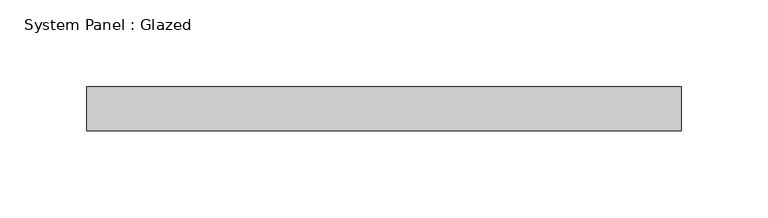
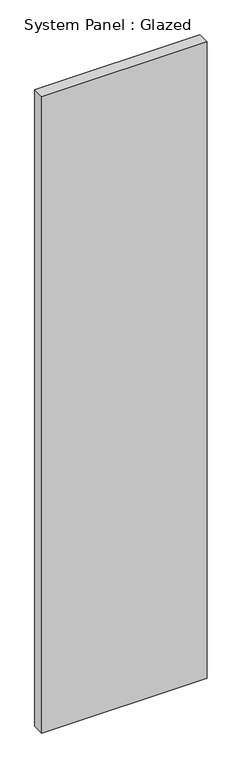
"""IFC4 building model written with IfcOpenShell, lengths in millimetres: plate geometry, System Panel : Glazed."""

from ifc_helpers import new_model, si_unit, origin, origin_with_axes, place, context, project, spatial, polyline, outline, extrude, source, transform, mapped, element, save


def system_panel_glazed_321d670a(model_context):
    return source(origin(), model_context, "Body", "SweptSolid", [
        extrude(outline(polyline([(171.45, 19.05), (-171.45, 19.05), (-171.45, 44.45), (171.45, 44.45), (171.45, 19.05)])), origin_with_axes(), (0.0, 0.0, 1.0), 1397.0),
    ])


if __name__ == "__main__":
    model = new_model("IFC4")
    model_context = context("Model", 3, world=origin())
    ifc_project = project(units=[si_unit("LENGTHUNIT", "METRE", prefix="MILLI")], contexts=[model_context])
    site = spatial("IfcSite", under=ifc_project)
    building = spatial("IfcBuilding", under=site)
    placement = place(None, origin())
    system_panel_glazed_shape = system_panel_glazed_321d670a(model_context)
    element("IfcPlate", 1, ObjectType="System Panel : Glazed", at=placement, inside=building, context=model_context, shape_type="MappedRepresentation", body=[
        mapped(system_panel_glazed_shape, transform((0.0, 0.0, 0.0), x_axis=(1.0, 0.0, 0.0), y_axis=(0.0, 1.0, 0.0), z_axis=(0.0, 0.0, 1.0))),
    ])
    save(model, "model.ifc")

# Revit data of these elements
# Type "System Panel : Glazed"
#   Construction Type Id = "GSP4R"
#   Analytic Construction = "1/8 in Pilkington single glazing"
#   Visual Light Transmittance = 0.9
#   Solar Heat Gain Coefficient = 0.86
#   Heat Transfer Coefficient (U) = 1.18115 BTU/(h·ft²·°F)
#   Define Thermal Properties by = 1
# Element 1 (IfcPlate, "System Panel : Glazed")
#   Materials on its faces: "Glass"
# Materials
#   "Glass": class "Glass", colour RGB 0 128 192, transparency 0.75, Description = "Soda Lime Glass", Cost = 0
